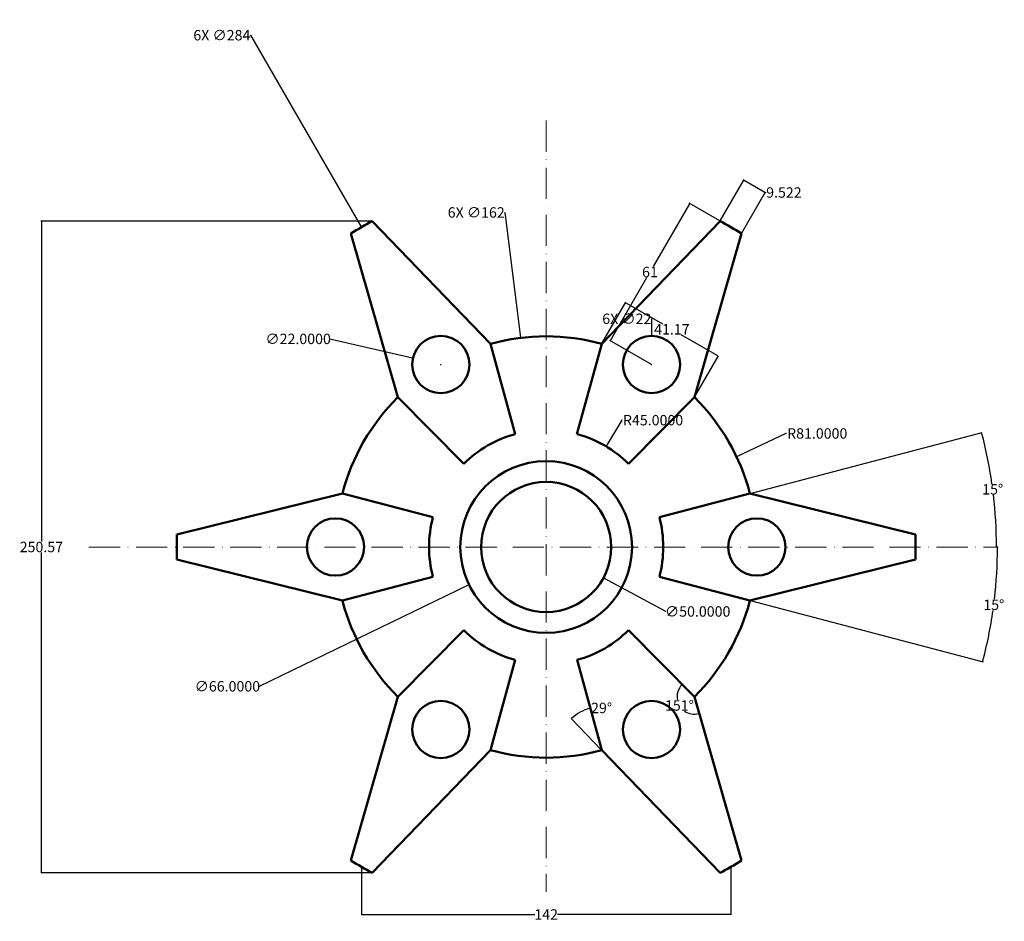
# Model space of a CAD drawing. Units: inches. Extents: x 458 to 836, y 348 to 695.
import ezdxf

# ---------------------------------------------------------------- set-up
doc = ezdxf.new("R2010")
doc.units = ezdxf.units.IN
doc.header["$MEASUREMENT"] = 0
doc.linetypes.add('ACAD_ISO10W100', pattern=[18, 12, -3, 0, -3])
for name, color, linetype, lineweight in [('M-CNTR', 4, 'ACAD_ISO10W100', 18), ('M-DIMS', 2, 'Continuous', 25), ('M-OUTL', 7, 'Continuous', 50)]:
    doc.layers.add(name, color=color, linetype=linetype, lineweight=lineweight)
doc.styles.get("Standard").update_dxf_attribs({"font": 'arial.ttf'})
doc.dimstyles.get("Standard").update_dxf_attribs({"dimtxt": 4, "dimasz": 0.18, "dimexe": 0.18, "dimexo": 0.0625, "dimgap": 0.09, "dimtad": 0, "dimtih": 1, "dimtoh": 1, "dimdec": 4, "dimzin": 0, "dimdsep": 46, "dimtxsty": 'Standard', "dimcen": 0.09, "dimadec": 0, "dimazin": 0, "dimtfac": 1, "dimtdec": 4, "dimtofl": 0, "dimtmove": 0, "dimatfit": 3, "dimfxl": 1, "dimtolj": 1, "dimtzin": 0, "dimarcsym": 0})

# ---------------------------------------------------------------- blocks, each defined once
blk = doc.blocks.new('*D1')
at = {"layer": 'Defpoints', "color": 0, "transparency": 16777216}
for p in [(682.94, 530.87), (659.9, 492.22)]:
    blk.add_point(p, dxfattribs=at)
at = {"layer": 'M-DIMS', "color": 0, "lineweight": -2, "transparency": 16777216}
for p, q in [((688.97, 540.98), (683.03, 531.03)), ((689.15, 540.98), (688.97, 540.98)), ((659.81, 492.22), (659.99, 492.22)), ((659.9, 492.13), (659.9, 492.31))]:
    blk.add_line(p, q, dxfattribs=at)
at = {"layer": 'M-DIMS', "color": 0, "transparency": 16777216}
blk.add_solid([(683.01, 531.04), (683.06, 531.01), (682.94, 530.87)], dxfattribs=at)
at = {"layer": 'M-DIMS', "color": 0, "transparency": 16777216, "insert": (701, 540.98), "char_height": 4, "attachment_point": 5}
blk.add_mtext('\\A1;R45.0000', dxfattribs=at)
blk = doc.blocks.new('*D2')
at = {"layer": 'Defpoints', "color": 0, "transparency": 16777216}
for p in [(733.11, 526.89), (659.9, 492.22)]:
    blk.add_point(p, dxfattribs=at)
at = {"layer": 'M-DIMS', "color": 0, "lineweight": -2, "transparency": 16777216}
for p, q in [((752.07, 535.87), (733.27, 526.96)), ((752.25, 535.87), (752.07, 535.87)), ((659.81, 492.22), (659.99, 492.22)), ((659.9, 492.13), (659.9, 492.31))]:
    blk.add_line(p, q, dxfattribs=at)
at = {"layer": 'M-DIMS', "color": 0, "transparency": 16777216}
blk.add_solid([(733.26, 526.99), (733.28, 526.94), (733.11, 526.89)], dxfattribs=at)
at = {"layer": 'M-DIMS', "color": 0, "transparency": 16777216, "insert": (764.1, 535.87), "char_height": 4, "attachment_point": 5}
blk.add_mtext('\\A1;R81.0000', dxfattribs=at)
blk = doc.blocks.new('*D3')
at = {"layer": 'Defpoints', "color": 0, "transparency": 16777216}
for p in [(608.68, 564.84), (630.12, 559.89)]:
    blk.add_point(p, dxfattribs=at)
at = {"layer": 'M-DIMS', "color": 0, "lineweight": -2, "transparency": 16777216}
for p, q in [((576.69, 572.22), (608.51, 564.88)), ((619.31, 562.36), (619.49, 562.36)), ((619.4, 562.27), (619.4, 562.45))]:
    blk.add_line(p, q, dxfattribs=at)
at = {"layer": 'M-DIMS', "color": 0, "transparency": 16777216}
blk.add_solid([(608.51, 564.91), (608.5, 564.85), (608.68, 564.84)], dxfattribs=at)
at = {"layer": 'M-DIMS', "color": 0, "transparency": 16777216, "insert": (564.57, 572.22), "char_height": 4, "attachment_point": 5}
blk.add_mtext('\\A1;∅22.0000', dxfattribs=at)
blk = doc.blocks.new('*D4')
at = {"layer": 'Defpoints', "color": 0, "transparency": 16777216}
for p in [(689.58, 506.63), (630.22, 477.8)]:
    blk.add_point(p, dxfattribs=at)
at = {"layer": 'M-DIMS', "color": 0, "lineweight": -2, "transparency": 16777216}
for p, q in [((659.81, 492.22), (659.99, 492.22)), ((659.9, 492.13), (659.9, 492.31)), ((549.66, 438.67), (630.05, 477.72)), ((549.48, 438.67), (549.66, 438.67))]:
    blk.add_line(p, q, dxfattribs=at)
at = {"layer": 'M-DIMS', "color": 0, "transparency": 16777216}
blk.add_solid([(630.04, 477.75), (630.07, 477.69), (630.22, 477.8)], dxfattribs=at)
at = {"layer": 'M-DIMS', "color": 0, "transparency": 16777216, "insert": (537.37, 438.67), "char_height": 4, "attachment_point": 5}
blk.add_mtext('\\A1;∅66.0000', dxfattribs=at)
blk = doc.blocks.new('*D5')
at = {"layer": 'Defpoints', "color": 0, "transparency": 16777216}
for p in [(637.9, 504.08), (681.9, 480.35)]:
    blk.add_point(p, dxfattribs=at)
at = {"layer": 'M-DIMS', "color": 0, "lineweight": -2, "transparency": 16777216}
for p, q in [((659.81, 492.22), (659.99, 492.22)), ((659.9, 492.13), (659.9, 492.31)), ((705.85, 467.43), (682.06, 480.26)), ((706.03, 467.43), (705.85, 467.43))]:
    blk.add_line(p, q, dxfattribs=at)
at = {"layer": 'M-DIMS', "color": 0, "transparency": 16777216}
blk.add_solid([(682.08, 480.29), (682.05, 480.24), (681.9, 480.35)], dxfattribs=at)
at = {"layer": 'M-DIMS', "color": 0, "transparency": 16777216, "insert": (718.15, 467.43), "char_height": 4, "attachment_point": 5}
blk.add_mtext('\\A1;∅50.0000', dxfattribs=at)
blk = doc.blocks.new('*D6')
at = {"layer": 'Defpoints', "color": 0, "transparency": 16777216}
for p in [(691.57, 460.24), (710.24, 434.06), (716.9, 434.66), (716.9, 434.66), (734.98, 371.69)]:
    blk.add_point(p, dxfattribs=at)
at = {"layer": 'M-DIMS', "color": 0, "lineweight": -2, "transparency": 16777216}
for start, end in [(136.2641, 190.7669), (235.5324, 284.4823)]:
    blk.add_arc((716.9, 434.66), 6.69, start, end, dxfattribs=at)
at = {"layer": 'M-DIMS', "color": 0, "transparency": 16777216}
for points in [[(712.04, 439.31), (712.09, 439.27), (712.19, 439.42)], [(718.56, 428.22), (718.58, 428.16), (718.74, 428.23)]]:
    blk.add_solid(points, dxfattribs=at)
at = {"layer": 'M-DIMS', "color": 0, "transparency": 16777216, "insert": (711.13, 431.28), "char_height": 4, "attachment_point": 5}
blk.add_mtext('\\A1;151°', dxfattribs=at)
blk = doc.blocks.new('*D7')
at = {"layer": 'Defpoints', "color": 0, "transparency": 16777216}
for p in [(671.76, 448.81), (671.75, 427.94), (681.24, 414.08), (681.24, 414.08), (726.74, 366.93)]:
    blk.add_point(p, dxfattribs=at)
at = {"layer": 'M-DIMS', "color": 0, "lineweight": -2, "transparency": 16777216}
for p, q in [((676.99, 430.33), (677.17, 430.33)), ((681.2, 414.12), (669.46, 426.3))]:
    blk.add_line(p, q, dxfattribs=at)
for start, end in [(105.892, 133.3616), (104.664, 105.278)]:
    blk.add_arc((681.24, 414.08), 16.8, start, end, dxfattribs=at)
at = {"layer": 'M-DIMS', "color": 0, "transparency": 16777216}
for points in [[(676.64, 430.26), (676.65, 430.2), (676.82, 430.28)], [(669.73, 426.27), (669.69, 426.31), (669.58, 426.17)]]:
    blk.add_solid(points, dxfattribs=at)
at = {"layer": 'M-DIMS', "color": 0, "transparency": 16777216, "insert": (681.22, 430.33), "char_height": 4, "attachment_point": 5}
blk.add_mtext('\\A1;29°', dxfattribs=at)
blk = doc.blocks.new('*D8')
at = {"layer": 'Defpoints', "color": 0, "transparency": 16777216}
for p in [(738.24, 512.8), (703.42, 503.65), (832.36, 507.02), (484.16, 492.22), (832.99, 492.22)]:
    blk.add_point(p, dxfattribs=at)
at = {"layer": 'M-DIMS', "color": 0, "lineweight": -2, "transparency": 16777216}
blk.add_line((738.3, 512.82), (827.48, 536.25), dxfattribs=at)
for start, end in [(8.0733, 14.6624), (0.0596, 6.6499)]:
    blk.add_arc((659.9, 492.22), 173.09, start, end, dxfattribs=at)
at = {"layer": 'M-DIMS', "color": 0, "transparency": 16777216}
for points in [[(827.33, 536.02), (827.38, 536.04), (827.31, 536.2)], [(833.02, 492.4), (832.96, 492.4), (832.99, 492.22)]]:
    blk.add_solid(points, dxfattribs=at)
at = {"layer": 'M-DIMS', "color": 0, "transparency": 16777216, "insert": (831.56, 514.39), "char_height": 4, "attachment_point": 5}
blk.add_mtext('\\A1;15°', dxfattribs=at)
blk = doc.blocks.new('*D9')
at = {"layer": 'Defpoints', "color": 0, "transparency": 16777216}
for p in [(484.16, 492.22), (832.99, 492.22), (703.42, 480.78), (738.24, 471.63), (830.87, 462.64)]:
    blk.add_point(p, dxfattribs=at)
at = {"layer": 'M-DIMS', "color": 0, "lineweight": -2, "transparency": 16777216}
for p, q in [((833.05, 492.22), (833.59, 492.22)), ((738.3, 471.62), (827.88, 448.08))]:
    blk.add_line(p, q, dxfattribs=at)
for start, end in [(353.3484, 359.9406), (345.3374, 351.9284)]:
    blk.add_arc((659.9, 492.22), 173.51, start, end, dxfattribs=at)
at = {"layer": 'M-DIMS', "color": 0, "transparency": 16777216}
for points in [[(833.38, 492.04), (833.44, 492.04), (833.41, 492.22)], [(827.78, 448.29), (827.73, 448.3), (827.71, 448.12)]]:
    blk.add_solid(points, dxfattribs=at)
at = {"layer": 'M-DIMS', "color": 0, "transparency": 16777216, "insert": (831.98, 469.99), "char_height": 4, "attachment_point": 5}
blk.add_mtext('\\A1;15°', dxfattribs=at)
blk = doc.blocks.new('HUB-ARM')
for p, q in [((0, 32.02), (34.82, 41.17)), ((34.82, 41.17), (98.4, 25.35)), ((34.82, 0), (98.4, 15.82)), ((0, 9.15), (34.82, 0))]:
    blk.add_line(p, q)
blk.add_circle((37.48, 20.58), 11)
for radius, start, end in [(45, 345.278, 14.722), (142, 358.0786, 1.9214)]:
    blk.add_arc((-43.52, 20.58), radius, start, end)
blk = doc.blocks.new('*D11')
at = {"layer": 'Defpoints', "color": 0, "transparency": 16777216}
for p in [(465.86, 617.5), (593.06, 617.5), (593.06, 366.93)]:
    blk.add_point(p, dxfattribs=at)
at = {"layer": 'M-DIMS', "color": 0, "lineweight": -2, "transparency": 16777216}
for p, q in [((593, 617.5), (465.68, 617.5)), ((465.86, 617.32), (465.86, 494.35)), ((465.86, 367.11), (465.86, 490.08)), ((593, 366.93), (465.68, 366.93))]:
    blk.add_line(p, q, dxfattribs=at)
at = {"layer": 'M-DIMS', "color": 0, "transparency": 16777216}
for points in [[(465.83, 617.32), (465.89, 617.32), (465.86, 617.5)], [(465.83, 367.11), (465.89, 367.11), (465.86, 366.93)]]:
    blk.add_solid(points, dxfattribs=at)
at = {"layer": 'M-DIMS', "color": 0, "transparency": 16777216, "insert": (465.86, 492.22), "char_height": 4, "attachment_point": 5}
blk.add_mtext('\\A1;250.57', dxfattribs=at)
blk = doc.blocks.new('*D12')
at = {"layer": 'Defpoints', "color": 0, "transparency": 16777216}
for p in [(588.9, 369.24), (730.9, 369.24), (588.9, 350.94)]:
    blk.add_point(p, dxfattribs=at)
at = {"layer": 'M-DIMS', "color": 0, "lineweight": -2, "transparency": 16777216}
for p, q in [((588.9, 369.18), (588.9, 350.76)), ((730.9, 369.18), (730.9, 350.76)), ((589.08, 350.94), (655.6, 350.94)), ((730.72, 350.94), (664.2, 350.94))]:
    blk.add_line(p, q, dxfattribs=at)
at = {"layer": 'M-DIMS', "color": 0, "transparency": 16777216}
for points in [[(589.08, 350.97), (589.08, 350.91), (588.9, 350.94)], [(730.72, 350.97), (730.72, 350.91), (730.9, 350.94)]]:
    blk.add_solid(points, dxfattribs=at)
at = {"layer": 'M-DIMS', "color": 0, "transparency": 16777216, "insert": (659.9, 350.94), "char_height": 4, "attachment_point": 5}
blk.add_mtext('\\A1;142', dxfattribs=at)
blk = doc.blocks.new('*D13')
at = {"layer": 'Defpoints', "color": 0, "transparency": 16777216}
for p in [(715.05, 624.34), (730.9, 615.19), (700.4, 562.36)]:
    blk.add_point(p, dxfattribs=at)
at = {"layer": 'M-DIMS', "color": 0, "lineweight": -2, "transparency": 16777216}
for p, q in [((714.96, 624.19), (701.03, 600.06)), ((730.85, 615.22), (714.9, 624.43)), ((684.64, 571.67), (698.57, 595.8)), ((700.35, 562.4), (684.4, 571.6))]:
    blk.add_line(p, q, dxfattribs=at)
at = {"layer": 'M-DIMS', "color": 0, "transparency": 16777216}
for points in [[(714.94, 624.2), (714.99, 624.17), (715.05, 624.34)], [(684.62, 571.68), (684.67, 571.65), (684.55, 571.51)]]:
    blk.add_solid(points, dxfattribs=at)
at = {"layer": 'M-DIMS', "color": 0, "transparency": 16777216, "insert": (699.8, 597.93), "char_height": 4, "attachment_point": 5}
blk.add_mtext('\\A1;61', dxfattribs=at)
blk = doc.blocks.new('*D14')
at = {"layer": 'Defpoints', "color": 0, "transparency": 16777216}
for p in [(681.24, 570.35), (726.05, 565.62), (716.9, 549.77)]:
    blk.add_point(p, dxfattribs=at)
at = {"layer": 'M-DIMS', "color": 0, "lineweight": -2, "transparency": 16777216}
for p, q in [((681.28, 570.41), (690.48, 586.36)), ((690.55, 586.11), (704.59, 578.01)), ((725.89, 565.71), (711.86, 573.81)), ((716.93, 549.82), (726.14, 565.77))]:
    blk.add_line(p, q, dxfattribs=at)
at = {"layer": 'M-DIMS', "color": 0, "transparency": 16777216}
for points in [[(690.57, 586.14), (690.54, 586.09), (690.39, 586.2)], [(725.91, 565.73), (725.88, 565.68), (726.05, 565.62)]]:
    blk.add_solid(points, dxfattribs=at)
at = {"layer": 'M-DIMS', "color": 0, "transparency": 16777216, "insert": (708.22, 575.91), "char_height": 4, "attachment_point": 5}
blk.add_mtext('\\A1;41.17', dxfattribs=at)
blk = doc.blocks.new('*D15')
at = {"layer": 'Defpoints', "color": 0, "transparency": 16777216}
for p in [(744.13, 628.59), (726.74, 617.5), (734.98, 612.74)]:
    blk.add_point(p, dxfattribs=at)
at = {"layer": 'M-DIMS', "color": 0, "lineweight": -2, "transparency": 16777216}
for p, q in [((726.77, 617.56), (735.98, 633.51)), ((736.04, 633.26), (743.98, 628.68)), ((735.02, 612.8), (744.22, 628.75)), ((744.13, 628.59), (744.29, 628.5)), ((744.29, 628.5), (744.47, 628.5))]:
    blk.add_line(p, q, dxfattribs=at)
at = {"layer": 'M-DIMS', "color": 0, "transparency": 16777216}
for points in [[(736.06, 633.29), (736.03, 633.24), (735.89, 633.35)], [(743.99, 628.71), (743.96, 628.65), (744.13, 628.59)]]:
    blk.add_solid(points, dxfattribs=at)
at = {"layer": 'M-DIMS', "color": 0, "transparency": 16777216, "insert": (751.29, 628.5), "char_height": 4, "attachment_point": 5}
blk.add_mtext('\\A1;9.522', dxfattribs=at)
blk = doc.blocks.new('*D16')
at = {"layer": 'Defpoints', "color": 0, "transparency": 16777216}
for p in [(588.9, 615.19), (730.9, 369.24)]:
    blk.add_point(p, dxfattribs=at)
at = {"layer": 'M-DIMS', "color": 0, "lineweight": -2, "transparency": 16777216}
for p, q in [((546.12, 688.98), (546.3, 688.98)), ((546.3, 688.98), (588.81, 615.35)), ((659.81, 492.22), (659.99, 492.22)), ((659.9, 492.13), (659.9, 492.31))]:
    blk.add_line(p, q, dxfattribs=at)
at = {"layer": 'M-DIMS', "color": 0, "transparency": 16777216}
blk.add_solid([(588.84, 615.36), (588.78, 615.33), (588.9, 615.19)], dxfattribs=at)
at = {"layer": 'M-DIMS', "color": 0, "transparency": 16777216, "insert": (535.24, 688.98), "char_height": 4, "attachment_point": 5}
blk.add_mtext('\\A1;6X ∅284', dxfattribs=at)
blk = doc.blocks.new('*D17')
at = {"layer": 'Defpoints', "color": 0, "transparency": 16777216}
for p in [(650, 572.61), (669.8, 411.82)]:
    blk.add_point(p, dxfattribs=at)
at = {"layer": 'M-DIMS', "color": 0, "lineweight": -2, "transparency": 16777216}
for p, q in [((643.88, 620.84), (644.06, 620.84)), ((644.06, 620.84), (649.98, 572.79)), ((659.81, 492.22), (659.99, 492.22)), ((659.9, 492.13), (659.9, 492.31))]:
    blk.add_line(p, q, dxfattribs=at)
at = {"layer": 'M-DIMS', "color": 0, "transparency": 16777216}
blk.add_solid([(650.01, 572.79), (649.95, 572.78), (650, 572.61)], dxfattribs=at)
at = {"layer": 'M-DIMS', "color": 0, "transparency": 16777216, "insert": (633.02, 620.84), "char_height": 4, "attachment_point": 5}
blk.add_mtext('\\A1;6X ∅162', dxfattribs=at)
blk = doc.blocks.new('*D18')
at = {"layer": 'Defpoints', "color": 0, "transparency": 16777216}
for p in [(700.4, 573.36), (700.4, 551.36)]:
    blk.add_point(p, dxfattribs=at)
at = {"layer": 'M-DIMS', "color": 0, "lineweight": -2, "transparency": 16777216}
for p, q in [((700.22, 579.96), (700.4, 579.96)), ((700.4, 579.96), (700.4, 573.54)), ((700.31, 562.36), (700.49, 562.36)), ((700.4, 562.27), (700.4, 562.45))]:
    blk.add_line(p, q, dxfattribs=at)
at = {"layer": 'M-DIMS', "color": 0, "transparency": 16777216}
blk.add_solid([(700.43, 573.54), (700.37, 573.54), (700.4, 573.36)], dxfattribs=at)
at = {"layer": 'M-DIMS', "color": 0, "transparency": 16777216, "insert": (690.91, 579.96), "char_height": 4, "attachment_point": 5}
blk.add_mtext('\\A1;6X ∅22', dxfattribs=at)

msp = doc.modelspace()

# ---------------------------------------------------------------- linework, layer by layer
at = {"layer": 'M-CNTR'}
for p, q in [((659.90068, 656.14932), (659.90068, 359.67547)), ((484.1616, 492.21581), (832.99137, 492.21581))]:
    msp.add_line(p, q, dxfattribs=at)
at = {"layer": 'M-OUTL'}
for radius in [33, 25]:
    msp.add_circle((659.90068, 492.21581), radius, dxfattribs=at)
for start, end in [(74.7220247, 105.2779753), (134.7220247, 165.2779753), (14.7220247, 45.2779753), (194.7220247, 225.2779753), (314.7220247, 345.2779753), (254.7220247, 285.2779753)]:
    msp.add_arc((659.90068, 492.21581), 81, start, end, dxfattribs=at)

# ---------------------------------------------------------------- block references
for p, rotation in [((655.96648, 540.19965), 120.0000000000002), ((699.4888, 519.61484), 60.0000000000001), ((616.37835, 512.80061), 180), ((620.31255, 464.81677), 239.9999999999999), ((663.83487, 444.23196), 300)]:
    msp.add_blockref('HUB-ARM', p, dxfattribs=dict(at, rotation=rotation))
msp.add_blockref('HUB-ARM', (703.423, 471.631), dxfattribs=at)

# ---------------------------------------------------------------- dimensions: what is measured, and where the dimension line sits
at = {"layer": 'M-DIMS'}
for p1, p2, picture, middle in [((730.90061, 369.24016), (588.90074, 615.19145), '*D16', (535.24224, 688.97684)), ((669.79995, 411.82299), (650.0014, 572.60862), '*D17', (633.01558, 620.84431)), ((700.40135, 551.36386), (700.4, 573.36386), '*D18', (690.90722, 579.96386))]:
    dim = msp.add_diameter_dim_2p(p1=p1, p2=p2, text='6X <>', dimstyle='Standard', override={"dimdec": 0, "dimlfac": 1, "dimrnd": 0, "dimzin": 0, "dimdsep": 46, "dimlunit": 2}, dxfattribs=at)
    dim.commit()
    dim.dimension.update_dxf_attribs({"geometry": picture, "text_midpoint": middle, "dimtype": 163})
for base, p1, p2, angle, override, picture, middle in [((744.13397, 628.59), (726.73754, 617.50281), (734.98397, 612.74173), 330, {"dimdec": 3, "dimlfac": 1, "dimrnd": 0, "dimzin": 0, "dimdsep": 46, "dimlunit": 2}, '*D15', (751.28837, 628.5)), ((715.05241, 624.34141), (700.40068, 562.36386), (730.90068, 615.19141), 60, {"dimdec": 0, "dimlfac": 1, "dimrnd": 0, "dimzin": 0, "dimdsep": 46, "dimlunit": 2}, '*D13', (699.80241, 597.92764)), ((465.8616, 617.50281), (593.06381, 366.9288), (593.06381, 617.50281), 90, {"dimdec": 2, "dimlfac": 1, "dimrnd": 0, "dimzin": 0, "dimdsep": 46, "dimlunit": 2}, '*D11', (465.8616, 492.2158)), ((726.04778, 565.61692), (681.24436, 570.35317), (716.89778, 549.76866), 330, {"dimdec": 2, "dimlfac": 1, "dimrnd": 0, "dimzin": 0, "dimdsep": 46, "dimlunit": 2}, '*D14', (708.22107, 575.90918)), ((588.90068, 350.9402), (730.90068, 369.2402), (588.90068, 369.2402), 180, {"dimdec": 0, "dimlfac": 1, "dimrnd": 0, "dimzin": 0, "dimdsep": 46, "dimlunit": 2}, '*D12', (659.90068, 350.9402))]:
    dim = msp.add_linear_dim(base=base, p1=p1, p2=p2, angle=angle, dimstyle='Standard', override=override, dxfattribs=at)
    dim.commit()
    dim.dimension.update_dxf_attribs({"geometry": picture, "text_midpoint": middle})
for p1, p2, picture, middle in [((630.11901, 559.89056), (608.68234, 564.83717), '*D3', (576.68939, 572.2197)), ((689.58453, 506.63347), (630.21683, 477.79814), '*D4', (537.36659, 438.67231)), ((637.89644, 504.08229), (681.90491, 480.34932), '*D5', (718.14812, 467.43498))]:
    dim = msp.add_diameter_dim_2p(p1=p1, p2=p2, dimstyle='Standard', override={"dimclrd": 0, "dimclre": 0, "dimclrt": 0}, dxfattribs=at)
    dim.commit()
    dim.dimension.update_dxf_attribs({"geometry": picture, "text_midpoint": middle, "dimtype": 163})
for mpoint, picture, middle in [((682.94026, 530.8704), '*D1', (700.99943, 540.97914)), ((733.1055, 526.88646), '*D2', (764.10141, 535.86705))]:
    dim = msp.add_radius_dim(center=(659.90068, 492.21581), mpoint=mpoint, dimstyle='Standard', override={"dimclrd": 0, "dimclre": 0, "dimclrt": 0}, dxfattribs=at)
    dim.commit()
    dim.dimension.update_dxf_attribs({"geometry": picture, "text_midpoint": middle, "dimtype": 164})
for base, line1, line2, picture, middle in [((832.35688, 507.02278), ((703.42333, 503.65164), (738.24146, 512.80031)), ((484.1616, 492.21581), (832.99137, 492.21581)), '*D8', (831.56485, 514.39232)), ((830.86677, 462.63971), ((484.1616, 492.21581), (832.99137, 492.21581)), ((703.42333, 480.77997), (738.24146, 471.6313)), '*D9', (831.97622, 469.98615)), ((710.23669, 434.06189), ((716.89778, 434.66295), (734.98397, 371.68988)), ((691.56573, 460.242), (716.89778, 434.66295)), '*D6', (711.12758, 431.28123)), ((671.75269, 427.93561), ((671.75828, 448.80616), (681.24436, 414.07844)), ((681.24436, 414.07844), (726.73754, 366.9288)), '*D7', (681.22012, 430.32756))]:
    dim = msp.add_angular_dim_2l(base=base, line1=line1, line2=line2, dimstyle='Standard', override={"dimclrd": 0, "dimclre": 0, "dimclrt": 0}, dxfattribs=at)
    dim.commit()
    dim.dimension.update_dxf_attribs({"geometry": picture, "text_midpoint": middle})

doc.saveas('drawing.dxf')
